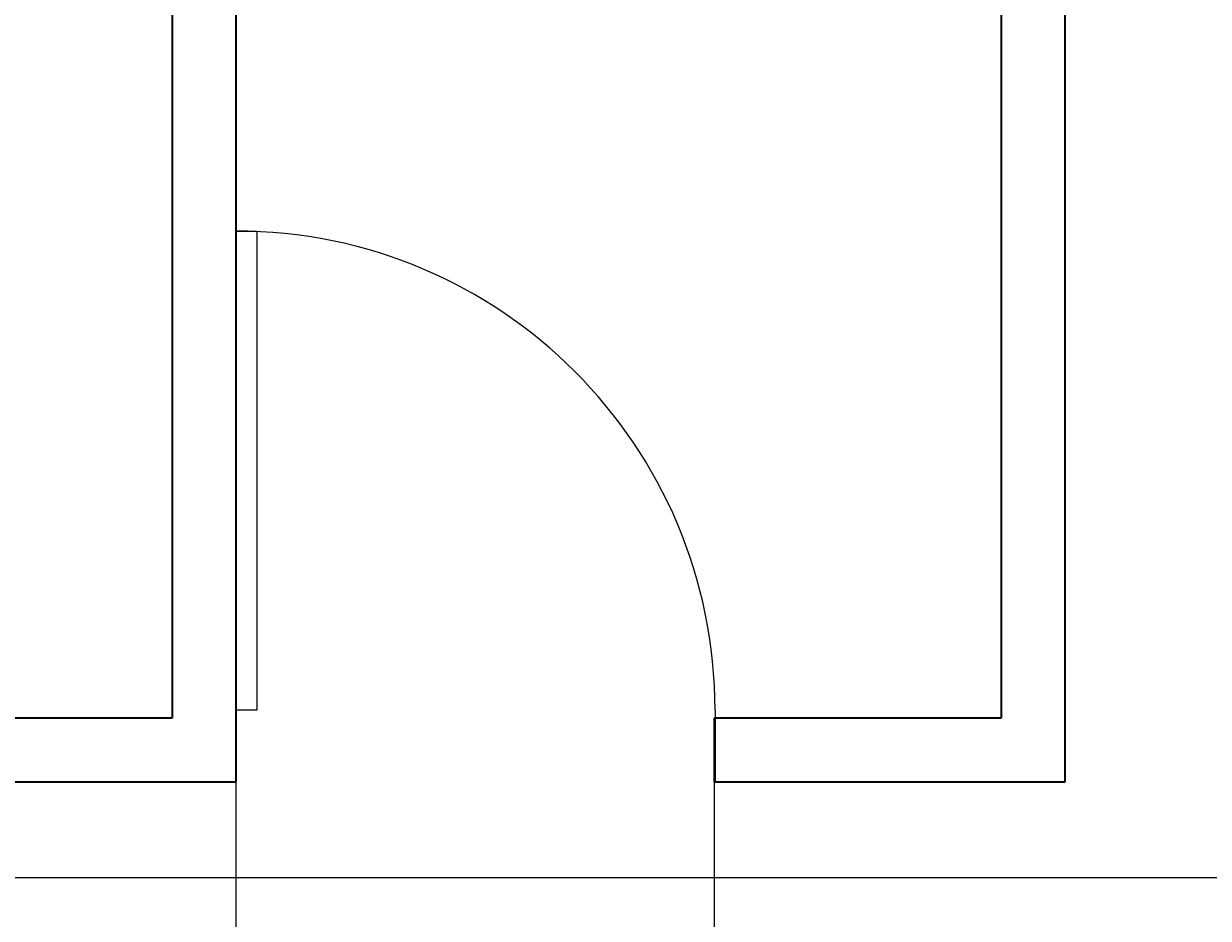
# Model space of a CAD drawing. Units: feet. Extents: x 105 to 1094, y -88 to 588.
# Tile 11 of 59: x 361 to 436, y 138 to 194. Entities that reach past the tile are written whole.
import ezdxf

# ---------------------------------------------------------------- set-up
doc = ezdxf.new("R2010")
doc.units = ezdxf.units.FT
doc.header["$MEASUREMENT"] = 0
for name, color, linetype, lineweight in [('A-ANNO-DIMS', 2, 'Continuous', 18), ('A-DOOR', 3, 'Continuous', 25), ('A-WALL', 7, 'Continuous', 35)]:
    doc.layers.add(name, color=color, linetype=linetype, lineweight=lineweight)
doc.styles.get("Standard").update_dxf_attribs({"font": 'arial.ttf'})
doc.dimstyles.get("Standard").update_dxf_attribs({"dimtxt": 0.18, "dimasz": 0.18, "dimexe": 0.18, "dimexo": 0.0625, "dimgap": 0.09, "dimtad": 0, "dimtih": 1, "dimtoh": 1, "dimdec": 4, "dimzin": 0, "dimdsep": 46, "dimtxsty": 'Standard', "dimcen": 0.09, "dimadec": 0, "dimazin": 0, "dimtfac": 1, "dimtdec": 4, "dimtofl": 0, "dimtmove": 0, "dimatfit": 3, "dimfxl": 1, "dimtolj": 1, "dimtzin": 0, "dimarcsym": 0})

# ---------------------------------------------------------------- blocks, each defined once
blk = doc.blocks.new('*U2')
for p, q in [((0, 0), (0, -6)), ((40, 0), (40, -6))]:
    blk.add_line(p, q)
blk.add_lwpolyline([(0, 0), (0, 40), (1.75, 40), (1.75, 0)], close=True)
blk.add_arc((0, 0), 40, 0, 90)
blk = doc.blocks.new('*D20')
at = {"layer": 'A-ANNO-DIMS', "color": 0, "lineweight": -2, "transparency": 16777216}
for p, q in [((150.688, 276.019), (150.688, -88.149)), ((1048.688, 276.019), (1048.688, -88.149)), ((150.868, -87.969), (599.399, -87.969)), ((1048.508, -87.969), (599.977, -87.969))]:
    blk.add_line(p, q, dxfattribs=at)
at = {"layer": 'A-ANNO-DIMS', "color": 0, "transparency": 16777216}
for points in [[(150.868, -87.939), (150.868, -87.999), (150.688, -87.969)], [(1048.508, -87.939), (1048.508, -87.999), (1048.688, -87.969)]]:
    blk.add_solid(points, dxfattribs=at)
at = {"layer": 'Defpoints', "color": 0, "transparency": 16777216}
for p in [(150.688, 276.081), (1048.688, 276.081), (1048.688, -87.969)]:
    blk.add_point(p, dxfattribs=at)
at = {"layer": 'A-ANNO-DIMS', "color": 0, "transparency": 16777216, "insert": (599.688, -87.969), "char_height": 0.18, "attachment_point": 5}
blk.add_mtext('\\A1;898', dxfattribs=at)
blk = doc.blocks.new('*D21')
at = {"layer": 'A-ANNO-DIMS', "color": 0, "lineweight": -2, "transparency": 16777216}
for p, q in [((849.626, 543.081), (105.458, 543.081)), ((105.638, 542.901), (105.638, 250.263)), ((105.638, -42.739), (105.638, 249.899)), ((849.626, -42.919), (105.458, -42.919))]:
    blk.add_line(p, q, dxfattribs=at)
at = {"layer": 'A-ANNO-DIMS', "color": 0, "transparency": 16777216}
for points in [[(105.608, 542.901), (105.668, 542.901), (105.638, 543.081)], [(105.608, -42.739), (105.668, -42.739), (105.638, -42.919)]]:
    blk.add_solid(points, dxfattribs=at)
at = {"layer": 'Defpoints', "color": 0, "transparency": 16777216}
for p in [(105.638, 543.081), (849.688, 543.081), (849.688, -42.919)]:
    blk.add_point(p, dxfattribs=at)
at = {"layer": 'A-ANNO-DIMS', "color": 0, "transparency": 16777216, "insert": (105.638, 250.081), "char_height": 0.18, "attachment_point": 5}
blk.add_mtext('\\A1;586', dxfattribs=at)
blk = doc.blocks.new('*D37')
at = {"layer": 'A-ANNO-DIMS', "color": 0, "lineweight": -2, "transparency": 16777216}
for p, q in [((374.688, 150.527), (374.688, -88.149)), ((404.688, 150.019), (404.688, -88.149)), ((374.868, -87.969), (389.47, -87.969)), ((404.508, -87.969), (389.907, -87.969))]:
    blk.add_line(p, q, dxfattribs=at)
at = {"layer": 'A-ANNO-DIMS', "color": 0, "transparency": 16777216}
for points in [[(374.868, -87.939), (374.868, -87.999), (374.688, -87.969)], [(404.508, -87.939), (404.508, -87.999), (404.688, -87.969)]]:
    blk.add_solid(points, dxfattribs=at)
at = {"layer": 'Defpoints', "color": 0, "transparency": 16777216}
for p in [(374.688, 150.59), (404.688, 150.081), (404.688, -87.969)]:
    blk.add_point(p, dxfattribs=at)
at = {"layer": 'A-ANNO-DIMS', "color": 0, "transparency": 16777216, "insert": (389.688, -87.969), "char_height": 0.18, "attachment_point": 5}
blk.add_mtext('\\A1;30', dxfattribs=at)
blk = doc.blocks.new('*D46')
at = {"layer": 'A-ANNO-DIMS', "color": 0, "lineweight": -2, "transparency": 16777216}
for p, q in [((580.626, 206.081), (105.458, 206.081)), ((105.638, 205.901), (105.638, 173.263)), ((105.638, 140.261), (105.638, 172.899)), ((580.626, 140.081), (105.458, 140.081))]:
    blk.add_line(p, q, dxfattribs=at)
at = {"layer": 'A-ANNO-DIMS', "color": 0, "transparency": 16777216}
for points in [[(105.608, 205.901), (105.668, 205.901), (105.638, 206.081)], [(105.608, 140.261), (105.668, 140.261), (105.638, 140.081)]]:
    blk.add_solid(points, dxfattribs=at)
at = {"layer": 'Defpoints', "color": 0, "transparency": 16777216}
for p in [(580.688, 206.081), (105.638, 140.081), (580.688, 140.081)]:
    blk.add_point(p, dxfattribs=at)
at = {"layer": 'A-ANNO-DIMS', "color": 0, "transparency": 16777216, "insert": (105.638, 173.081), "char_height": 0.18, "attachment_point": 5}
blk.add_mtext('\\A1;66', dxfattribs=at)

msp = doc.modelspace()

# ---------------------------------------------------------------- linework, layer by layer
at = {"layer": 'A-WALL'}
for p, q in [((374.6883, 248.0812), (374.6883, 146.0812)), ((422.6883, 248.0812), (422.6883, 150.0812)), ((426.6883, 248.0812), (426.6883, 146.0812)), ((370.6883, 198.0812), (370.6883, 150.0812)), ((370.6883, 150.0812), (288.6883, 150.0812)), ((422.6883, 150.0812), (404.6883, 150.0812)), ((404.6883, 150.0812), (404.6883, 146.0812)), ((374.6883, 146.0812), (288.6883, 146.0812)), ((426.6883, 146.0812), (404.6883, 146.0812))]:
    msp.add_line(p, q, dxfattribs=at)

# ---------------------------------------------------------------- block references
at = {"layer": 'A-DOOR', "xscale": 0.7513941790917756, "yscale": 0.7513941790917756, "zscale": 0.7513941790917756}
msp.add_blockref('*U2', (374.6883, 150.5895), dxfattribs=at)

# ---------------------------------------------------------------- dimensions: what is measured, and where the dimension line sits
at = {"layer": 'A-ANNO-DIMS'}
for base, p1, p2, picture, middle in [((105.6383, 543.0812), (849.6883, -42.9188), (849.6883, 543.0812), '*D21', (105.6383, 250.0812)), ((105.6383, 140.0812), (580.6883, 206.0812), (580.6883, 140.0812), '*D46', (105.6383, 173.0812))]:
    dim = msp.add_linear_dim(base=base, p1=p1, p2=p2, angle=90, dimstyle='Standard', override={"dimdec": 0, "dimlfac": 1, "dimrnd": 0, "dimzin": 0, "dimdsep": 46, "dimlunit": 2}, dxfattribs=at)
    dim.commit()
    dim.dimension.update_dxf_attribs({"geometry": picture, "text_midpoint": middle})
for base, p1, p2, picture, middle in [((1048.6883, -87.9688), (150.6883, 276.0812), (1048.6883, 276.0812), '*D20', (599.6883, -87.9688)), ((404.6883, -87.9688), (374.6883, 150.5895), (404.6883, 150.0812), '*D37', (389.6883, -87.9688))]:
    dim = msp.add_linear_dim(base=base, p1=p1, p2=p2, dimstyle='Standard', override={"dimdec": 0, "dimlfac": 1, "dimrnd": 0, "dimzin": 0, "dimdsep": 46, "dimlunit": 2}, dxfattribs=at)
    dim.commit()
    dim.dimension.update_dxf_attribs({"geometry": picture, "text_midpoint": middle})

doc.saveas('drawing.dxf')
